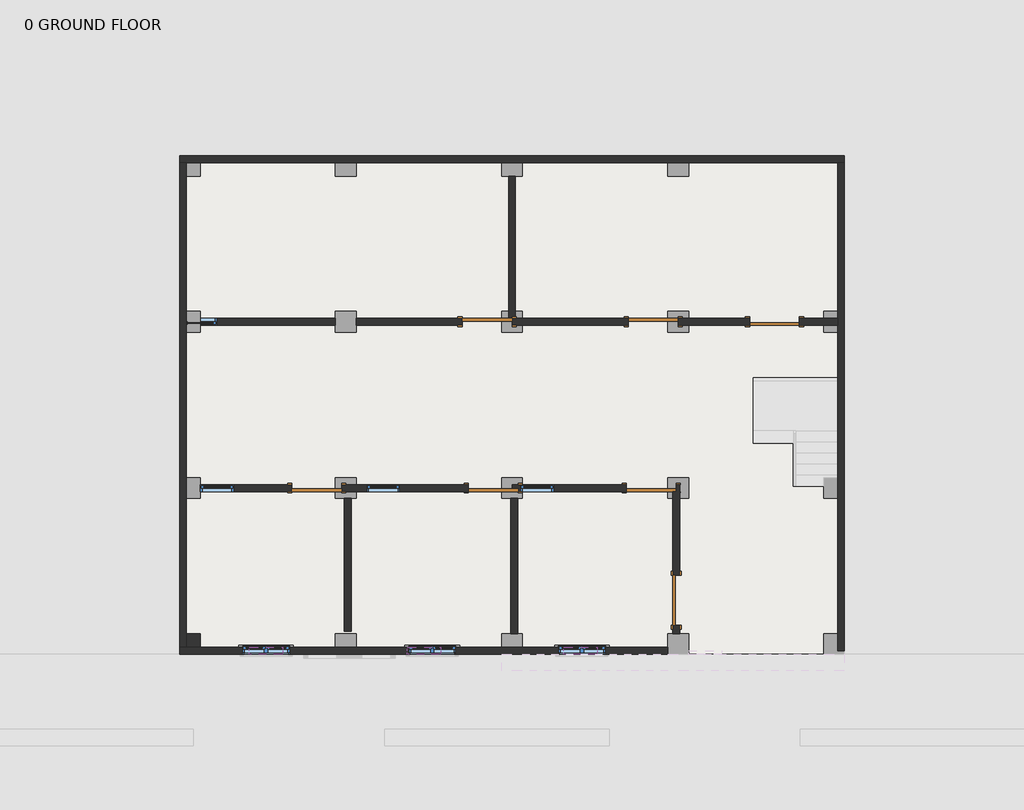
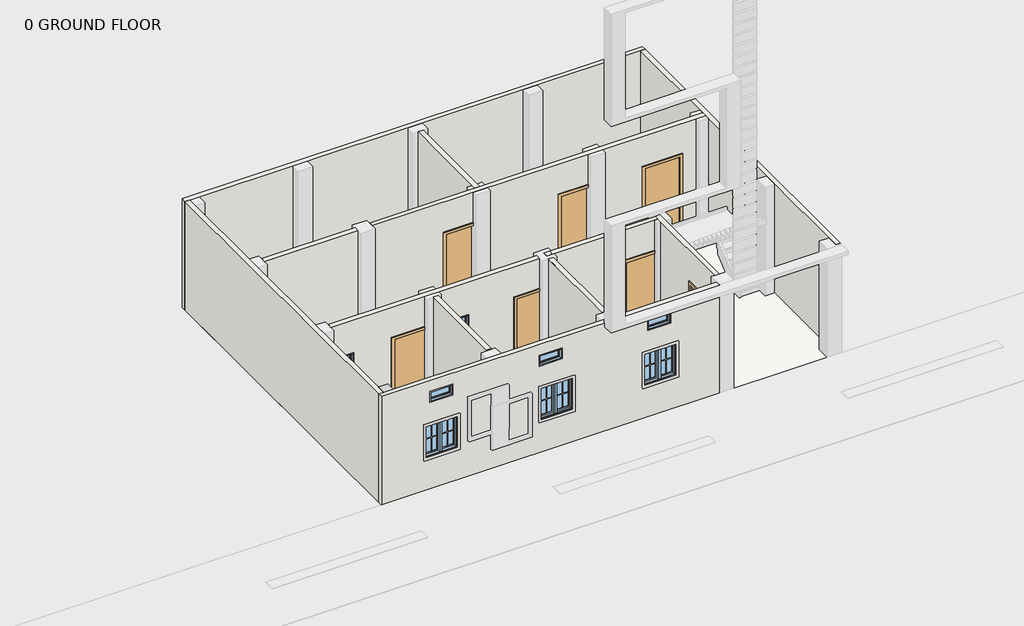
# One storey, part 1 of 2: 14 walls, 10 windows, 7 doors, 1 column, 1 slab.
"""IFC4 building model written with IfcOpenShell, lengths in millimetres."""

from ifc_helpers import new_model, si_unit, frame, origin, origin_with_axes, place, context, project, spatial, polyline, outline, extrude, faceted_brep, transform, mapped, element, save
from components import door_a1797ceb, window_4c2727af, window_0bf3737e, window_78893e6c, window_0d9958e7

model = new_model("IFC4")

# Units and contexts
model_context = context("Model", 3, world=origin())
ifc_project = project(units=[si_unit("LENGTHUNIT", "METRE", prefix="MILLI")], contexts=[model_context])

# Site, building, storey
site = spatial("IfcSite", under=ifc_project)
building = spatial("IfcBuilding", under=site)
storey = spatial("IfcBuildingStorey", under=building, Name="0 GROUND FLOOR", Elevation=0.0)

# Column
placement = place(None, origin())
element("IfcColumn", 1, ObjectType="column family : column family", at=placement, inside=storey, context=model_context, shape_type="SweptSolid", body=[
    extrude(outline(polyline([(-15433.597125, 9.7065522), (-15433.597125, -244.2934478), (-15687.597125, -244.2934478), (-15687.597125, 9.7065522), (-15433.597125, 9.7065522)])), frame((0.0, 0.0, 5.0), z_axis=(0.0, 0.0, 1.0), x_axis=(1.0, 0.0, 0.0)), (0.0, 0.0, 1.0), 3038.0),
])

# Doors
door_shape = door_a1797ceb(model_context)
element("IfcDoor", 2, ObjectType="Single-Flush : 36\" x 84\"", at=placement, inside=storey, context=model_context, shape_type="MappedRepresentation", body=[
    mapped(door_shape, transform((-10175.797125, 5724.7065522, 0.0), x_axis=(1.0, 0.0, 0.0), y_axis=(0.0, 1.0, 0.0), z_axis=(0.0, 0.0, 1.0))),
])
element("IfcDoor", 3, ObjectType="Single-Flush : 36\" x 84\"", at=placement, inside=storey, context=model_context, shape_type="MappedRepresentation", body=[
    mapped(door_shape, transform((-10061.497125, 2676.7065522, 0.0), x_axis=(-1.0, 0.0, 0.0), y_axis=(0.0, -1.0, 0.0), z_axis=(0.0, 0.0, 1.0))),
])
element("IfcDoor", 4, ObjectType="Single-Flush : 36\" x 84\"", at=placement, inside=storey, context=model_context, shape_type="MappedRepresentation", body=[
    mapped(door_shape, transform((-13299.997125, 2676.7065522, 0.0), x_axis=(-1.0, 0.0, 0.0), y_axis=(0.0, -1.0, 0.0), z_axis=(0.0, 0.0, 1.0))),
])
element("IfcDoor", 5, ObjectType="Single-Flush : 36\" x 84\"", at=placement, inside=storey, context=model_context, shape_type="MappedRepresentation", body=[
    mapped(door_shape, transform((-7127.797125, 5724.7065522, 0.0), x_axis=(1.0, 0.0, 0.0), y_axis=(0.0, 1.0, 0.0), z_axis=(0.0, 0.0, 1.0))),
])
element("IfcDoor", 6, ObjectType="Single-Flush : 36\" x 84\"", at=placement, inside=storey, context=model_context, shape_type="MappedRepresentation", body=[
    mapped(door_shape, transform((-7165.897125, 2676.7065522, 0.0), x_axis=(-1.0, 0.0, 0.0), y_axis=(0.0, -1.0, 0.0), z_axis=(0.0, 0.0, 1.0))),
])
element("IfcDoor", 7, ObjectType="Single-Flush : 36\" x 84\"", at=placement, inside=storey, context=model_context, shape_type="MappedRepresentation", body=[
    mapped(door_shape, transform((-6708.697125, 619.3065522, 0.0), x_axis=(0.0, 1.0, 0.0), y_axis=(-1.0, 0.0, 0.0), z_axis=(0.0, 0.0, 1.0))),
])
element("IfcDoor", 8, ObjectType="Single-Flush : 36\" x 84\"", at=placement, inside=storey, context=model_context, shape_type="MappedRepresentation", body=[
    mapped(door_shape, transform((-4905.297125, 5724.7065522, 0.0), x_axis=(-1.0, 0.0, 0.0), y_axis=(0.0, -1.0, 0.0), z_axis=(0.0, 0.0, 1.0))),
])

# Slab
element("IfcSlab", 9, ObjectType="Generic - 4\"", at=placement, inside=storey, context=model_context, shape_type="SweptSolid", body=[
    extrude(outline(polyline([(-3622.597125, 8772.7065522), (-3622.597125, -371.2934478), (-15814.597125, -371.2934478), (-15814.597125, 8772.7065522), (-3622.597125, 8772.7065522)])), frame((0.0, 0.0, -101.6), z_axis=(0.0, 0.0, 1.0), x_axis=(1.0, 0.0, 0.0)), (0.0, 0.0, 1.0), 101.6),
])

# Walls
element("IfcWall", 10, ObjectType="Generic - 5\"", at=placement, inside=storey, context=model_context, shape_type="Brep", body=[
    faceted_brep([(-15814.597125, 8645.7065522, 0.0), (-15687.597125, 8645.7065522, 0.0), (-3749.597125, 8645.7065522, 0.0), (-3622.597125, 8645.7065522, 0.0), (-3622.597125, 8645.7065522, 3048.0), (-3749.597125, 8645.7065522, 3048.0), (-15687.597125, 8645.7065522, 3048.0), (-15814.597125, 8645.7065522, 3048.0), (-15814.597125, 8772.7065522, 0.0), (-15814.597125, 8772.7065522, 3048.0), (-3622.597125, 8772.7065522, 3048.0), (-3622.597125, 8772.7065522, 0.0)], [[[0, 1, 2, 3, 4, 5, 6, 7]], [[8, 9, 10, 11]], [[3, 2, 1, 0, 8, 11]], [[7, 6, 5, 4, 10, 9]], [[4, 3, 11, 10]], [[0, 7, 9, 8]]]),
])
element("IfcWall", 11, ObjectType="Generic - 5\"", at=placement, inside=storey, context=model_context, shape_type="Brep", body=[
    faceted_brep([(-3749.597125, 8645.7065522, 0.0), (-3749.597125, 5788.2065522, 0.0), (-3749.597125, 5661.2065522, 0.0), (-3749.597125, -307.7934478, 0.0), (-3749.597125, -307.7934478, 5.0), (-3749.597125, -307.7934478, 3043.0), (-3749.597125, -307.7934478, 3048.0), (-3749.597125, 5661.2065522, 3048.0), (-3749.597125, 5788.2065522, 3048.0), (-3749.597125, 8645.7065522, 3048.0), (-3622.597125, 8645.7065522, 0.0), (-3622.597125, 8645.7065522, 3048.0), (-3622.597125, -307.7934478, 3048.0), (-3622.597125, -307.7934478, 3043.0), (-3622.597125, -307.7934478, 5.0), (-3622.597125, -307.7934478, 0.0)], [[[0, 1, 2, 3, 4, 5, 6, 7, 8, 9]], [[10, 11, 12, 13, 14, 15]], [[3, 2, 1, 0, 10, 15]], [[6, 5, 4, 3, 15, 14, 13, 12]], [[9, 8, 7, 6, 12, 11]], [[0, 9, 11, 10]]]),
])
element("IfcWall", 12, ObjectType="Generic - 5\"", at=placement, inside=storey, context=model_context, shape_type="Brep", body=[
    faceted_brep([(-6861.097125, -244.2934478, 0.0), (-15687.597125, -244.2934478, 0.0), (-15814.597125, -244.2934478, 0.0), (-15814.597125, -244.2934478, 3048.0), (-15687.597125, -244.2934478, 3048.0), (-6861.097125, -244.2934478, 3048.0), (-13795.297125, -244.2934478, 1828.8), (-14658.897125, -244.2934478, 1828.8), (-14658.897125, -244.2934478, 914.4), (-13795.297125, -244.2934478, 914.4), (-10747.297125, -244.2934478, 1828.8), (-11610.897125, -244.2934478, 1828.8), (-11610.897125, -244.2934478, 914.4), (-10747.297125, -244.2934478, 914.4), (-8004.097125, -244.2934478, 1828.8), (-8867.697125, -244.2934478, 1828.8), (-8867.697125, -244.2934478, 914.4), (-8004.097125, -244.2934478, 914.4), (-13922.297125, -244.2934478, 2743.2), (-14531.897125, -244.2934478, 2743.2), (-14531.897125, -244.2934478, 2438.4), (-13922.297125, -244.2934478, 2438.4), (-11026.697125, -244.2934478, 2743.2), (-11636.297125, -244.2934478, 2743.2), (-11636.297125, -244.2934478, 2438.4), (-11026.697125, -244.2934478, 2438.4), (-8156.497125, -244.2934478, 2743.2), (-8766.097125, -244.2934478, 2743.2), (-8766.097125, -244.2934478, 2438.4), (-8156.497125, -244.2934478, 2438.4), (-6861.097125, -371.2934478, 0.0), (-6861.097125, -371.2934478, 5.0), (-6861.097125, -371.2934478, 3043.0), (-6861.097125, -371.2934478, 3048.0), (-15814.597125, -371.2934478, 3048.0), (-15814.597125, -371.2934478, 0.0), (-13795.297125, -371.2934478, 1828.8), (-13795.297125, -371.2934478, 914.4), (-14658.897125, -371.2934478, 914.4), (-14658.897125, -371.2934478, 1828.8), (-10747.297125, -371.2934478, 1828.8), (-10747.297125, -371.2934478, 914.4), (-11610.897125, -371.2934478, 914.4), (-11610.897125, -371.2934478, 1828.8), (-8004.097125, -371.2934478, 1828.8), (-8004.097125, -371.2934478, 914.4), (-8867.697125, -371.2934478, 914.4), (-8867.697125, -371.2934478, 1828.8), (-13922.297125, -371.2934478, 2743.2), (-13922.297125, -371.2934478, 2438.4), (-14531.897125, -371.2934478, 2438.4), (-14531.897125, -371.2934478, 2743.2), (-11026.697125, -371.2934478, 2743.2), (-11026.697125, -371.2934478, 2438.4), (-11636.297125, -371.2934478, 2438.4), (-11636.297125, -371.2934478, 2743.2), (-8156.497125, -371.2934478, 2743.2), (-8156.497125, -371.2934478, 2438.4), (-8766.097125, -371.2934478, 2438.4), (-8766.097125, -371.2934478, 2743.2)], [[[0, 1, 2, 3, 4, 5], [6, 7, 8, 9], [10, 11, 12, 13], [14, 15, 16, 17], [18, 19, 20, 21], [22, 23, 24, 25], [26, 27, 28, 29]], [[30, 31, 32, 33, 34, 35], [36, 37, 38, 39], [40, 41, 42, 43], [44, 45, 46, 47], [48, 49, 50, 51], [52, 53, 54, 55], [56, 57, 58, 59]], [[2, 1, 0, 30, 35]], [[5, 4, 3, 34, 33]], [[0, 5, 33, 32, 31, 30]], [[3, 2, 35, 34]], [[37, 36, 6, 9]], [[38, 37, 9, 8]], [[39, 38, 8, 7]], [[36, 39, 7, 6]], [[41, 40, 10, 13]], [[42, 41, 13, 12]], [[43, 42, 12, 11]], [[40, 43, 11, 10]], [[45, 44, 14, 17]], [[46, 45, 17, 16]], [[47, 46, 16, 15]], [[44, 47, 15, 14]], [[49, 48, 18, 21]], [[50, 49, 21, 20]], [[51, 50, 20, 19]], [[48, 51, 19, 18]], [[53, 52, 22, 25]], [[54, 53, 25, 24]], [[55, 54, 24, 23]], [[52, 55, 23, 22]], [[57, 56, 26, 29]], [[58, 57, 29, 28]], [[59, 58, 28, 27]], [[56, 59, 27, 26]]]),
])
element("IfcWall", 13, ObjectType="Generic - 5\"", at=placement, inside=storey, context=model_context, shape_type="Brep", body=[
    faceted_brep([(-15687.597125, -244.2934478, 0.0), (-15687.597125, 8645.7065522, 0.0), (-15687.597125, 8645.7065522, 5.0), (-15687.597125, 8645.7065522, 3043.0), (-15687.597125, 8645.7065522, 3048.0), (-15687.597125, -244.2934478, 3048.0), (-15687.597125, -244.2934478, 3043.0), (-15687.597125, -244.2934478, 5.0), (-15814.597125, -244.2934478, 0.0), (-15814.597125, -244.2934478, 3048.0), (-15814.597125, 8645.7065522, 3048.0), (-15814.597125, 8645.7065522, 0.0)], [[[0, 1, 2, 3, 4, 5, 6, 7]], [[8, 9, 10, 11]], [[1, 0, 8, 11]], [[5, 4, 10, 9]], [[4, 3, 2, 1, 11, 10]], [[0, 7, 6, 5, 9, 8]]]),
])
element("IfcWall", 14, ObjectType="Generic - 5\"", at=placement, inside=storey, context=model_context, shape_type="SweptSolid", body=[
    extrude(outline(polyline([(0.0, -15433.597125), (0.0, -12957.097125), (3048.0, -12957.097125), (3048.0, -15433.597125), (2133.6, -15433.597125), (2133.6, -15128.797125), (304.8, -15128.797125), (304.8, -15433.597125), (0.0, -15433.597125)])), frame((0.0, 5661.2065522, 0.0), z_axis=(0.0, 1.0, 0.0), x_axis=(0.0, 0.0, 1.0)), (0.0, 0.0, 1.0), 127.0),
])
element("IfcWall", 15, ObjectType="Generic - 5\"", at=placement, inside=storey, context=model_context, shape_type="Brep", body=[
    faceted_brep([(-9782.097125, 8391.7065522, 0.0), (-9782.097125, 5788.2065522, 0.0), (-9782.097125, 5788.2065522, 5.0), (-9782.097125, 5788.2065522, 2133.6), (-9782.097125, 5788.2065522, 3043.0), (-9782.097125, 5788.2065522, 3048.0), (-9782.097125, 8391.7065522, 3048.0), (-9655.097125, 8391.7065522, 0.0), (-9655.097125, 8391.7065522, 3048.0), (-9655.097125, 5788.2065522, 3048.0), (-9655.097125, 5788.2065522, 3043.0), (-9655.097125, 5788.2065522, 5.0), (-9655.097125, 5788.2065522, 0.0)], [[[0, 1, 2, 3, 4, 5, 6]], [[7, 8, 9, 10, 11, 12]], [[1, 0, 7, 12]], [[6, 5, 9, 8]], [[0, 6, 8, 7]], [[5, 4, 3, 2, 1, 12, 11, 10, 9]]]),
])
element("IfcWall", 16, ObjectType="Generic - 5\"", at=placement, inside=storey, context=model_context, shape_type="Brep", body=[
    faceted_brep([(-6670.597125, 5661.2065522, 0.0), (-5362.497125, 5661.2065522, 0.0), (-5362.497125, 5661.2065522, 2133.6), (-4448.097125, 5661.2065522, 2133.6), (-4448.097125, 5661.2065522, 0.0), (-3749.597125, 5661.2065522, 0.0), (-3749.597125, 5661.2065522, 5.0), (-3749.597125, 5661.2065522, 3043.0), (-3749.597125, 5661.2065522, 3048.0), (-12576.097125, 5661.2065522, 3048.0), (-12576.097125, 5661.2065522, 0.0), (-10632.997125, 5661.2065522, 0.0), (-10632.997125, 5661.2065522, 2133.6), (-9909.097125, 5661.2065522, 2133.6), (-9718.597125, 5661.2065522, 2133.6), (-9718.597125, 5661.2065522, 5.0), (-9718.597125, 5661.2065522, 0.0), (-7584.997125, 5661.2065522, 0.0), (-7584.997125, 5661.2065522, 2133.6), (-6861.097125, 5661.2065522, 2133.6), (-6670.597125, 5661.2065522, 2133.6), (-6670.597125, 5661.2065522, 5.0), (-5362.497125, 5788.2065522, 2133.6), (-5362.497125, 5788.2065522, 0.0), (-6670.597125, 5788.2065522, 0.0), (-6670.597125, 5788.2065522, 5.0), (-6670.597125, 5788.2065522, 2133.6), (-6861.097125, 5788.2065522, 2133.6), (-7584.997125, 5788.2065522, 2133.6), (-7584.997125, 5788.2065522, 0.0), (-9655.097125, 5788.2065522, 0.0), (-9718.597125, 5788.2065522, 0.0), (-9718.597125, 5788.2065522, 5.0), (-9718.597125, 5788.2065522, 2133.6), (-9782.097125, 5788.2065522, 2133.6), (-9909.097125, 5788.2065522, 2133.6), (-10632.997125, 5788.2065522, 2133.6), (-10632.997125, 5788.2065522, 0.0), (-12576.097125, 5788.2065522, 0.0), (-12576.097125, 5788.2065522, 3048.0), (-9782.097125, 5788.2065522, 3048.0), (-9655.097125, 5788.2065522, 3048.0), (-3749.597125, 5788.2065522, 3048.0), (-3749.597125, 5788.2065522, 3043.0), (-3749.597125, 5788.2065522, 5.0), (-3749.597125, 5788.2065522, 0.0), (-4448.097125, 5788.2065522, 0.0), (-4448.097125, 5788.2065522, 2133.6)], [[[0, 1, 2, 3, 4, 5, 6, 7, 8, 9, 10, 11, 12, 13, 14, 15, 16, 17, 18, 19, 20, 21]], [[22, 23, 24, 25, 26, 27, 28, 29, 30, 31, 32, 33, 34, 35, 36, 37, 38, 39, 40, 41, 42, 43, 44, 45, 46, 47]], [[11, 10, 38, 37]], [[17, 16, 31, 30, 29]], [[46, 45, 5, 4]], [[24, 23, 1, 0]], [[9, 8, 42, 41, 40, 39]], [[10, 9, 39, 38]], [[8, 7, 6, 5, 45, 44, 43, 42]], [[33, 32, 31, 16, 15, 14]], [[36, 35, 34, 33, 14, 13, 12]], [[37, 36, 12, 11]], [[26, 25, 24, 0, 21, 20]], [[28, 27, 26, 20, 19, 18]], [[29, 28, 18, 17]], [[2, 1, 23, 22]], [[3, 2, 22, 47]], [[4, 3, 47, 46]]]),
])
element("IfcWall", 17, ObjectType="Generic - 5\"", at=placement, inside=storey, context=model_context, shape_type="Brep", body=[
    faceted_brep([(-14823.997125, 2613.2065522, 304.8), (-15433.597125, 2613.2065522, 304.8), (-15433.597125, 2613.2065522, 0.0), (-13757.197125, 2613.2065522, 0.0), (-13757.197125, 2613.2065522, 2133.6), (-12957.097125, 2613.2065522, 2133.6), (-12842.797125, 2613.2065522, 2133.6), (-12842.797125, 2613.2065522, 5.0), (-12842.797125, 2613.2065522, 0.0), (-10518.697125, 2613.2065522, 0.0), (-10518.697125, 2613.2065522, 2133.6), (-9909.097125, 2613.2065522, 2133.6), (-9909.097125, 2613.2065522, 3048.0), (-15433.597125, 2613.2065522, 3048.0), (-15433.597125, 2613.2065522, 2133.6), (-14823.997125, 2613.2065522, 2133.6), (-12385.597125, 2613.2065522, 2133.6), (-11775.997125, 2613.2065522, 2133.6), (-11775.997125, 2613.2065522, 304.8), (-12385.597125, 2613.2065522, 304.8), (-15433.597125, 2740.2065522, 0.0), (-15433.597125, 2740.2065522, 304.8), (-14823.997125, 2740.2065522, 304.8), (-14823.997125, 2740.2065522, 2133.6), (-15433.597125, 2740.2065522, 2133.6), (-15433.597125, 2740.2065522, 3048.0), (-9909.097125, 2740.2065522, 3048.0), (-9909.097125, 2740.2065522, 2133.6), (-10518.697125, 2740.2065522, 2133.6), (-10518.697125, 2740.2065522, 0.0), (-12842.797125, 2740.2065522, 0.0), (-12842.797125, 2740.2065522, 5.0), (-12842.797125, 2740.2065522, 2133.6), (-12957.097125, 2740.2065522, 2133.6), (-13757.197125, 2740.2065522, 2133.6), (-13757.197125, 2740.2065522, 0.0), (-12385.597125, 2740.2065522, 2133.6), (-12385.597125, 2740.2065522, 304.8), (-11775.997125, 2740.2065522, 304.8), (-11775.997125, 2740.2065522, 2133.6)], [[[0, 1, 2, 3, 4, 5, 6, 7, 8, 9, 10, 11, 12, 13, 14, 15], [16, 17, 18, 19]], [[20, 21, 22, 23, 24, 25, 26, 27, 28, 29, 30, 31, 32, 33, 34, 35], [36, 37, 38, 39]], [[30, 29, 9, 8]], [[20, 35, 3, 2]], [[26, 12, 11, 27]], [[13, 12, 26, 25]], [[14, 13, 25, 24]], [[2, 1, 21, 20]], [[28, 10, 9, 29]], [[10, 28, 27, 11]], [[4, 3, 35, 34]], [[6, 5, 4, 34, 33, 32]], [[8, 7, 6, 32, 31, 30]], [[22, 21, 1, 0]], [[23, 22, 0, 15]], [[24, 23, 15, 14]], [[37, 36, 16, 19]], [[38, 37, 19, 18]], [[39, 38, 18, 17]], [[36, 39, 17, 16]]]),
])
element("IfcWall", 18, ObjectType="Generic - 5\"", at=placement, inside=storey, context=model_context, shape_type="SweptSolid", body=[
    extrude(outline(polyline([(-9616.997125, 2486.2065522), (-9616.997125, 9.7065522), (-9743.997125, 9.7065522), (-9743.997125, 2486.2065522), (-9616.997125, 2486.2065522)])), origin_with_axes(), (0.0, 0.0, 1.0), 3048.0),
])
element("IfcWall", 19, ObjectType="Generic - 5\"", at=placement, inside=storey, context=model_context, shape_type="SweptSolid", body=[
    extrude(outline(polyline([(-9743.997125, 2181.4065522), (-9743.997125, 2486.2065522), (-9616.997125, 2486.2065522), (-9616.997125, 2181.4065522), (-9743.997125, 2181.4065522)])), origin_with_axes(), (0.0, 0.0, 1.0), 3048.0),
])
element("IfcWall", 20, ObjectType="Generic - 5\"", at=placement, inside=storey, context=model_context, shape_type="Brep", body=[
    faceted_brep([(-6772.197125, 2613.2065522, 3048.0), (-9718.597125, 2613.2065522, 3048.0), (-9718.597125, 2613.2065522, 3043.0), (-9718.597125, 2613.2065522, 5.0), (-9718.597125, 2613.2065522, 0.0), (-7623.097125, 2613.2065522, 0.0), (-7623.097125, 2613.2065522, 2133.6), (-6861.097125, 2613.2065522, 2133.6), (-6772.197125, 2613.2065522, 2133.6), (-6772.197125, 2613.2065522, 3043.0), (-9566.197125, 2613.2065522, 2133.6), (-9528.097125, 2613.2065522, 2133.6), (-8956.597125, 2613.2065522, 2133.6), (-8956.597125, 2613.2065522, 304.8), (-9528.097125, 2613.2065522, 304.8), (-9566.197125, 2613.2065522, 304.8), (-9718.597125, 2740.2065522, 3048.0), (-6772.197125, 2740.2065522, 3048.0), (-6772.197125, 2740.2065522, 2133.6), (-6861.097125, 2740.2065522, 2133.6), (-7623.097125, 2740.2065522, 2133.6), (-7623.097125, 2740.2065522, 0.0), (-9718.597125, 2740.2065522, 0.0), (-9718.597125, 2740.2065522, 5.0), (-9718.597125, 2740.2065522, 3043.0), (-9566.197125, 2740.2065522, 2133.6), (-9566.197125, 2740.2065522, 304.8), (-9528.097125, 2740.2065522, 304.8), (-8956.597125, 2740.2065522, 304.8), (-8956.597125, 2740.2065522, 2133.6), (-9528.097125, 2740.2065522, 2133.6)], [[[0, 1, 2, 3, 4, 5, 6, 7, 8, 9], [10, 11, 12, 13, 14, 15]], [[16, 17, 18, 19, 20, 21, 22, 23, 24], [25, 26, 27, 28, 29, 30]], [[4, 22, 21, 5]], [[1, 0, 17, 16]], [[4, 3, 2, 1, 16, 24, 23, 22]], [[26, 25, 10, 15]], [[28, 27, 26, 15, 14, 13]], [[29, 28, 13, 12]], [[25, 30, 29, 12, 11, 10]], [[20, 6, 5, 21]], [[6, 20, 19, 18, 8, 7]], [[17, 0, 9, 8, 18]]]),
])
element("IfcWall", 21, ObjectType="Generic - 5\"", at=placement, inside=storey, context=model_context, shape_type="Brep", body=[
    faceted_brep([(-6645.197125, 2740.2065522, 3048.0), (-6645.197125, 9.7065522, 3048.0), (-6645.197125, 9.7065522, 0.0), (-6645.197125, 162.1065522, 0.0), (-6645.197125, 162.1065522, 2133.6), (-6645.197125, 1076.5065522, 2133.6), (-6645.197125, 1076.5065522, 0.0), (-6645.197125, 2740.2065522, 0.0), (-6645.197125, 2740.2065522, 5.0), (-6645.197125, 2740.2065522, 3043.0), (-6772.197125, 9.7065522, 3048.0), (-6772.197125, 2613.2065522, 3048.0), (-6772.197125, 2740.2065522, 3048.0), (-6772.197125, 2740.2065522, 2133.6), (-6772.197125, 2613.2065522, 2133.6), (-6772.197125, 2613.2065522, 5.0), (-6772.197125, 2613.2065522, 0.0), (-6772.197125, 1076.5065522, 0.0), (-6772.197125, 1076.5065522, 2133.6), (-6772.197125, 162.1065522, 2133.6), (-6772.197125, 162.1065522, 0.0), (-6772.197125, 9.7065522, 0.0), (-6708.697125, 2613.2065522, 0.0), (-6708.697125, 2740.2065522, 0.0), (-6708.697125, 2613.2065522, 2133.6), (-6708.697125, 2613.2065522, 5.0), (-6708.697125, 2740.2065522, 2133.6), (-6708.697125, 2740.2065522, 5.0)], [[[0, 1, 2, 3, 4, 5, 6, 7, 8, 9]], [[10, 11, 12, 13, 14, 15, 16, 17, 18, 19, 20, 21]], [[2, 21, 20, 3]], [[7, 6, 17, 16, 22, 23]], [[1, 0, 12, 11, 10]], [[2, 1, 10, 21]], [[5, 18, 17, 6]], [[18, 5, 4, 19]], [[24, 25, 22, 16, 15, 14]], [[26, 24, 14, 13]], [[22, 25, 24, 26, 27, 23]], [[0, 9, 8, 7, 23, 27, 26, 13, 12]], [[19, 4, 3, 20]]]),
])
element("IfcWall", 22, ObjectType="Generic - 5\"", at=placement, inside=storey, context=model_context, shape_type="Brep", body=[
    faceted_brep([(-9718.597125, 2613.2065522, 0.0), (-9566.197125, 2613.2065522, 0.0), (-9566.197125, 2613.2065522, 304.8), (-9566.197125, 2613.2065522, 2133.6), (-9566.197125, 2613.2065522, 3048.0), (-9718.597125, 2613.2065522, 3048.0), (-9718.597125, 2613.2065522, 3043.0), (-9718.597125, 2613.2065522, 5.0), (-9718.597125, 2740.2065522, 0.0), (-9718.597125, 2740.2065522, 5.0), (-9718.597125, 2740.2065522, 3043.0), (-9718.597125, 2740.2065522, 3048.0), (-9566.197125, 2740.2065522, 3048.0), (-9566.197125, 2740.2065522, 2133.6), (-9566.197125, 2740.2065522, 304.8), (-9566.197125, 2740.2065522, 0.0)], [[[0, 1, 2, 3, 4, 5, 6, 7]], [[8, 9, 10, 11, 12, 13, 14, 15]], [[1, 0, 8, 15]], [[4, 3, 2, 1, 15, 14, 13, 12]], [[5, 4, 12, 11]], [[0, 7, 6, 5, 11, 10, 9, 8]]]),
])
element("IfcWall", 23, ObjectType="Generic - 5\"", at=placement, inside=storey, context=model_context, shape_type="SweptSolid", body=[
    extrude(outline(polyline([(-12791.997125, 47.8065522), (-12791.997125, 2486.2065522), (-12664.997125, 2486.2065522), (-12664.997125, 47.8065522), (-12791.997125, 47.8065522)])), origin_with_axes(), (0.0, 0.0, 1.0), 3048.0),
])

# Windows
window_shape = window_4c2727af(model_context)
element("IfcWindow", 24, ObjectType="Fixed : 24\" x 12\"", at=placement, inside=storey, context=model_context, shape_type="MappedRepresentation", body=[
    mapped(window_shape, transform((-14188.997125, -307.7934478, 1524.0), x_axis=(1.0, 0.0, 0.0), y_axis=(0.0, 1.0, 0.0), z_axis=(0.0, 0.0, 1.0))),
])
element("IfcWindow", 25, ObjectType="Fixed : 24\" x 12\"", at=placement, inside=storey, context=model_context, shape_type="MappedRepresentation", body=[
    mapped(window_shape, transform((-11293.397125, -307.7934478, 1524.0), x_axis=(1.0, 0.0, 0.0), y_axis=(0.0, 1.0, 0.0), z_axis=(0.0, 0.0, 1.0))),
])
element("IfcWindow", 26, ObjectType="Fixed : 24\" x 12\"", at=placement, inside=storey, context=model_context, shape_type="MappedRepresentation", body=[
    mapped(window_shape, transform((-8423.197125, -307.7934478, 1524.0), x_axis=(1.0, 0.0, 0.0), y_axis=(0.0, 1.0, 0.0), z_axis=(0.0, 0.0, 1.0))),
])
window_2_shape = window_0bf3737e(model_context)
element("IfcWindow", 27, ObjectType="Fixed : 24\" x 72\"", at=placement, inside=storey, context=model_context, shape_type="MappedRepresentation", body=[
    mapped(window_2_shape, transform((-15471.697125, 5724.7065522, 0.0), x_axis=(-1.0, 0.0, 0.0), y_axis=(0.0, -1.0, 0.0), z_axis=(0.0, 0.0, 1.0))),
])
window_3_shape = window_78893e6c(model_context)
element("IfcWindow", 28, ObjectType="Fixed : 24\" x 72\"", at=placement, inside=storey, context=model_context, shape_type="MappedRepresentation", body=[
    mapped(window_3_shape, transform((-15166.897125, 2676.7065522, 0.0), x_axis=(-1.0, 0.0, 0.0), y_axis=(0.0, -1.0, 0.0), z_axis=(0.0, 0.0, 1.0))),
])
element("IfcWindow", 29, ObjectType="Fixed : 24\" x 72\"", at=placement, inside=storey, context=model_context, shape_type="MappedRepresentation", body=[
    mapped(window_3_shape, transform((-12118.897125, 2676.7065522, 0.0), x_axis=(-1.0, 0.0, 0.0), y_axis=(0.0, -1.0, 0.0), z_axis=(0.0, 0.0, 1.0))),
])
element("IfcWindow", 30, ObjectType="Fixed : 24\" x 72\"", at=placement, inside=storey, context=model_context, shape_type="MappedRepresentation", body=[
    mapped(window_3_shape, transform((-9299.497125, 2676.7065522, 0.0), x_axis=(-1.0, 0.0, 0.0), y_axis=(0.0, -1.0, 0.0), z_axis=(0.0, 0.0, 1.0))),
])
window_4_shape = window_0d9958e7(model_context)
element("IfcWindow", 31, ObjectType="Window-Casement-Double : 34\" x 36\"", at=placement, inside=storey, context=model_context, shape_type="MappedRepresentation", body=[
    mapped(window_4_shape, transform((-14227.097125, -307.7934478, 0.0), x_axis=(1.0, 0.0, 0.0), y_axis=(0.0, 1.0, 0.0), z_axis=(0.0, 0.0, 1.0))),
])
element("IfcWindow", 32, ObjectType="Window-Casement-Double : 34\" x 36\"", at=placement, inside=storey, context=model_context, shape_type="MappedRepresentation", body=[
    mapped(window_4_shape, transform((-11179.097125, -307.7934478, 0.0), x_axis=(1.0, 0.0, 0.0), y_axis=(0.0, 1.0, 0.0), z_axis=(0.0, 0.0, 1.0))),
])
element("IfcWindow", 33, ObjectType="Window-Casement-Double : 34\" x 36\"", at=placement, inside=storey, context=model_context, shape_type="MappedRepresentation", body=[
    mapped(window_4_shape, transform((-8435.897125, -307.7934478, 0.0), x_axis=(1.0, 0.0, 0.0), y_axis=(0.0, 1.0, 0.0), z_axis=(0.0, 0.0, 1.0))),
])

save(model, "model.ifc")

# Revit data of these elements
# Grids (mm)
#   "1": line (-15814.597, -3654.63) -> (-15814.597, 8772.707)
#   "2": line (-12766.597, -3654.63) -> (-12766.597, 8772.707)
#   "3": line (-9718.597, -3654.63) -> (-9718.597, 8772.707)
#   "4": line (-6670.597, -3654.63) -> (-6670.597, 8772.707)
#   "5": line (-3622.597, -3654.63) -> (-3622.597, 8772.707)
#   "6": line (-2073.402, 8772.707) -> (-15814.597, 8772.707)
#   "7": line (-2073.402, 5724.707) -> (-15814.597, 5724.707)
#   "8": line (-2073.402, 2676.707) -> (-15814.597, 2676.707)
#   "9": line (-2073.402, -371.293) -> (-15814.597, -371.293)
# Type "column family : column family"
#   w2 [instance default] = 0' - 9.88189"
#   w1 [instance default] = 0' - 9.01575"
#   Depth = 1' - 11.62205"
#   Width = 1' - 11.62205"
# Type "Single-Flush : 36\" x 84\""
#   Type Mark = "1"
#   Construction Type Id = "MDOOR"
#   Assembly Code = "C1020"
#   Analytic Construction = "Metal"
#   Thickness = 0' - 2"
#   Heat Transfer Coefficient (U) = 0.651978 BTU/(h·ft²·°F)
#   Height = 7' - 0"
#   Trim Projection Ext = 0' - 1"
#   Trim Projection Int = 0' - 1"
#   Trim Width = 0' - 3"
#   Width = 3' - 0"
#   Define Thermal Properties by = 1
#   Define Thermal Properties by = 1
#   Door Material = Door - Panel
#   Frame Material = Door - Frame
#   Visual Light Transmittance = 0
#   Solar Heat Gain Coefficient = 0
#   Function = (empty or 0)
#   Wall Closure = (empty or 0)
# Type "Generic - 4\""
#   Assembly Code = "B1010"
#   Function = 0
#   Layers, outside or top first: 0' - 4" no material (function 1)
# Type "Generic - 5\""
#   Assembly Code = "B2010"
#   Layers, outside or top first: 0' - 5" no material (function 1)
# Type "Fixed : 24\" x 12\""
#   Type Mark = "4"
#   Construction Type Id = "GSP4R"
#   Assembly Code = "B2020100"
#   Analytic Construction = "1/8 in Pilkington single glazing"
#   Visual Light Transmittance = 0.9
#   Solar Heat Gain Coefficient = 0.78
#   Heat Transfer Coefficient (U) = 0.6496 BTU/(h·ft²·°F)
#   Height = 1' - 0"
#   Default Sill Height = 3' - 0"
#   Width = 2' - 0"
#   Window Inset = 0' - 0 3/4"
#   Define Thermal Properties by = 1
#   Define Thermal Properties by = 1
#   Glass Pane Material = Glass
#   Sash Material = Sash
#   Wall Closure = (empty or 0)
# Type "Fixed : 24\" x 72\""
#   Type Mark = "7"
#   Construction Type Id = "GSP4R"
#   Assembly Code = "B2020100"
#   Analytic Construction = "1/8 in Pilkington single glazing"
#   Visual Light Transmittance = 0.9
#   Solar Heat Gain Coefficient = 0.78
#   Heat Transfer Coefficient (U) = 0.6496 BTU/(h·ft²·°F)
#   Height = 6' - 0"
#   Default Sill Height = 1' - 0"
#   Width = 2' - 0"
#   Window Inset = 0' - 0 3/4"
#   Define Thermal Properties by = 1
#   Define Thermal Properties by = 1
#   Glass Pane Material = Glass
#   Sash Material = Sash
#   Wall Closure = (empty or 0)
# Type "Window-Casement-Double : 34\" x 36\""
#   Type Mark = "14"
#   Fire Rating = "0.5h"
#   Assembly Code = "B2020100"
#   Analytic Construction = "Double glazing - domestic"
#   Frame Extension [instance default] = 0' - 0 1/4"
#   Window Inset [instance default] = 0' - 0"
#   Wall Thickness [instance default] = 0' - 6"
#   Interior Wall Closure [instance default] = 0' - 2 1/4"
#   Half Width = 1' - 5"
#   Visual Light Transmittance = 0.81
#   Thermal Resistance (R) = 1.8146 (h·ft²·°F)/BTU
#   Solar Heat Gain Coefficient = 0.76
#   Rough Width = 2' - 10 1/2"
#   Rough Height = 3' - 0 1/2"
#   Height = 3' - 0"
#   Heat Transfer Coefficient (U) = 0.5511 BTU/(h·ft²·°F)
#   Exterior Wall Closure [instance default] = 0' - 1 1/4"
#   Extension Jamb [instance default] = 0' - 2 1/4"
#   Default Sill Height = 3' - 0"
#   Width = 2' - 10"
#   Define Thermal Properties by = 0
#   Muntin Visibility = yes
#   Interior Trim Visibility [instance default] = yes
#   Exterior Trim Visibility [instance default] = yes
#   Extension Jamb Visibility [instance default] = yes
#   Interior Trim Material = Wood - Stained
#   Muntin Pattern = Muntin Pattern_2x2 : Muntin Pattern_2x2
#   Interior Trim = Trim-Window-Interior-Flat : Picture Frame
#   Interior Frame Material = Wood - Stained
#   Glass Panel Material = Glass
#   Exterior Trim Material = Clad - White
#   Exterior Trim = Trim-Window-Exterior-Flat : with Sill
#   Exterior Frame Material = Clad - White
#   Wall Closure = (empty or 0)
# Element 1 (IfcColumn, "column family : column family")
#   w2 = 1' - 3"
#   w1 = 1' - 3"
#   Phase Created = New Construction
#   Materials on its faces: "Default Wall"
# Elements 2, 3, 4, 5, 6, 7, 8 (IfcDoor, "Single-Flush : 36\" x 84\"")
#   Phase Created = New Construction
#   Materials on its faces: "Door - Frame", "Door - Panel"
# Element 9 (IfcSlab, "Generic - 4\"")
#   Height Offset From Level = 0' - 0"
#   Phase Created = New Construction
#   Materials on its faces: "Default Floor", "Clad - White", "floor"
# Element 10 (IfcWall, "Generic - 5\"")
#   Top Offset = 0' - 0"
#   Base Offset = 0' - 0"
#   wall height = 10' - 0"
#   Phase Created = New Construction
#   Base Constraint = 0 GROUND FLOOR
#   Top Constraint = 1st FLOOR
#   Materials on its faces: "Default Wall", "Clad - White"
# Element 11 (IfcWall, "Generic - 5\"")
#   Top Offset = 0' - 0"
#   Base Offset = 0' - 0"
#   wall height = 10' - 0"
#   Phase Created = New Construction
#   Base Constraint = 0 GROUND FLOOR
#   Top Constraint = 1st FLOOR
#   Materials on its faces: "Default Wall", "grey", "Clad - White"
# Element 12 (IfcWall, "Generic - 5\"")
#   Top Offset = 0' - 0"
#   Base Offset = 0' - 0"
#   wall height = 10' - 0"
#   Phase Created = New Construction
#   Base Constraint = 0 GROUND FLOOR
#   Top Constraint = 1st FLOOR
#   Materials on its faces: "Default Wall", "out side wall", "Clad - White"
# Element 13 (IfcWall, "Generic - 5\"")
#   Top Offset = 0' - 0"
#   Base Offset = 0' - 0"
#   wall height = 10' - 0"
#   Phase Created = New Construction
#   Base Constraint = 0 GROUND FLOOR
#   Top Constraint = 1st FLOOR
#   Materials on its faces: "Default Wall", "inside wall", "Clad - White"
# Elements 14, 17, 20 (IfcWall, "Generic - 5\"")
#   Top Offset = 0' - 0"
#   Base Offset = 0' - 0"
#   wall height = 10' - 0"
#   Phase Created = New Construction
#   Base Constraint = 0 GROUND FLOOR
#   Top Constraint = 1st FLOOR
#   Materials on its faces: "Default Wall", "inside wall"
# Elements 15, 18, 19, 22, 23 (IfcWall, "Generic - 5\"")
#   Top Offset = 0' - 0"
#   Base Offset = 0' - 0"
#   wall height = 10' - 0"
#   Phase Created = New Construction
#   Base Constraint = 0 GROUND FLOOR
#   Top Constraint = 1st FLOOR
#   Materials on its faces: "Default Wall"
# Element 16 (IfcWall, "Generic - 5\"")
#   Top Offset = 0' - 0"
#   Base Offset = 0' - 0"
#   wall height = 10' - 0"
#   Phase Created = New Construction
#   Base Constraint = 0 GROUND FLOOR
#   Top Constraint = 1st FLOOR
#   Materials on its faces: "Default Wall", "grey"
# Element 21 (IfcWall, "Generic - 5\"")
#   Top Offset = 0' - 0"
#   Base Offset = 0' - 0"
#   wall height = 10' - 0"
#   Phase Created = New Construction
#   Base Constraint = 0 GROUND FLOOR
#   Top Constraint = 1st FLOOR
#   Materials on its faces: "Default Wall", "grey", "inside wall"
# Element 24 (IfcWindow, "Fixed : 24\" x 12\"")
#   Mark = "12"
#   Phase Created = New Construction
#   Materials on its faces: "Sash", "Glass"
# Element 25 (IfcWindow, "Fixed : 24\" x 12\"")
#   Mark = "13"
#   Phase Created = New Construction
#   Materials on its faces: "Sash", "Glass"
# Element 26 (IfcWindow, "Fixed : 24\" x 12\"")
#   Mark = "14"
#   Phase Created = New Construction
#   Materials on its faces: "Sash", "Glass"
# Element 27 (IfcWindow, "Fixed : 24\" x 72\"")
#   Mark = "2"
#   Phase Created = New Construction
#   Materials on its faces: "Sash", "Glass"
# Element 28 (IfcWindow, "Fixed : 24\" x 72\"")
#   Mark = "3"
#   Phase Created = New Construction
#   Materials on its faces: "Sash", "Glass"
# Element 29 (IfcWindow, "Fixed : 24\" x 72\"")
#   Mark = "4"
#   Phase Created = New Construction
#   Materials on its faces: "Sash", "Glass"
# Element 30 (IfcWindow, "Fixed : 24\" x 72\"")
#   Mark = "5"
#   Phase Created = New Construction
#   Materials on its faces: "Sash", "Glass"
# Element 31 (IfcWindow, "Window-Casement-Double : 34\" x 36\"")
#   Mark = "8"
#   Window Inset = 0' - 0"
#   Interior Wall Closure = 0' - 2 1/4"
#   Frame Extension = 0' - 0 1/4"
#   Exterior Wall Closure = 0' - 1 1/4"
#   Interior Trim Visibility = yes
#   Exterior Trim Visibility = yes
#   Phase Created = New Construction
#   Materials on its faces: "Wood - Stained", "Glass", "Clad - White"
# Element 32 (IfcWindow, "Window-Casement-Double : 34\" x 36\"")
#   Mark = "9"
#   Window Inset = 0' - 0"
#   Interior Wall Closure = 0' - 2 1/4"
#   Frame Extension = 0' - 0 1/4"
#   Exterior Wall Closure = 0' - 1 1/4"
#   Interior Trim Visibility = yes
#   Exterior Trim Visibility = yes
#   Phase Created = New Construction
#   Materials on its faces: "Wood - Stained", "Glass", "Clad - White"
# Element 33 (IfcWindow, "Window-Casement-Double : 34\" x 36\"")
#   Mark = "11"
#   Window Inset = 0' - 0"
#   Interior Wall Closure = 0' - 2 1/4"
#   Frame Extension = 0' - 0 1/4"
#   Exterior Wall Closure = 0' - 1 1/4"
#   Interior Trim Visibility = yes
#   Exterior Trim Visibility = yes
#   Phase Created = New Construction
#   Materials on its faces: "Wood - Stained", "Glass", "Clad - White"
# Materials
#   "Door - Panel": class "Wood", colour RGB 210 159 95, transparency 0, Cost = 0
#   "Door - Frame": colour RGB 118 70 51, transparency 0, Cost = 0
#   "Glass": class "Glass", colour RGB 0 128 192, transparency 0.75, Description = "Soda Lime Glass", Cost = 0
#   "Sash": class "Wood", colour RGB 224 178 126, transparency 0, Cost = 0
#   "Wood - Stained": class "Wood", colour RGB 224 178 126, transparency 0, Cost = 0
#   "Clad - White": class "Wood", colour RGB 242 242 238, transparency 0, Cost = 0
#   "Default Wall": colour RGB 128 128 128, transparency 0, Cost = 0
#   "Default Floor": colour RGB 128 128 128, transparency 0, Cost = 0
#   "floor": class "Generic", colour RGB 255 255 255, transparency 0, Cost = 0
#   "grey": class "Generic", colour RGB 80 80 80, transparency 0, Cost = 0
#   "out side wall": class "Generic", colour RGB 16 106 159, transparency 0, Cost = 0
#   "inside wall": class "Generic", colour RGB 199 224 95, transparency 0, Cost = 0
